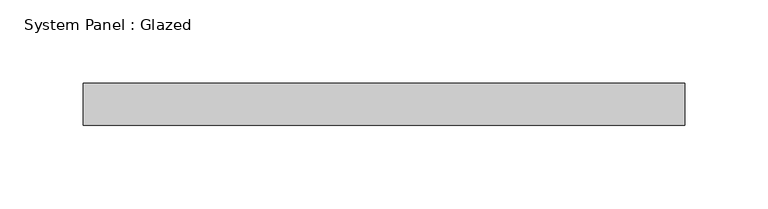
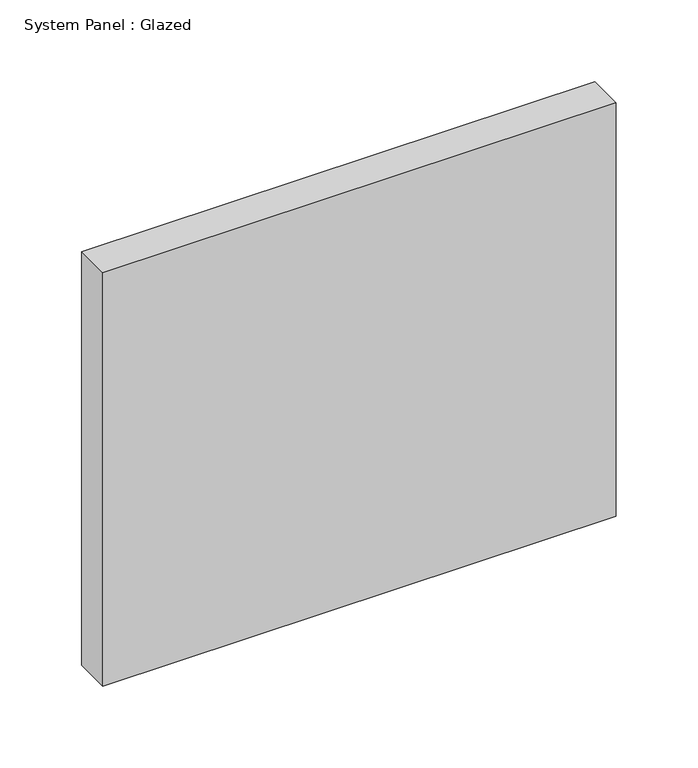
"""IFC4 building model written with IfcOpenShell, lengths in millimetres: plate geometry, System Panel : Glazed."""

from ifc_helpers import new_model, si_unit, origin, origin_with_axes, place, context, project, spatial, polyline, outline, extrude, source, transform, mapped, element, save


def system_panel_glazed_bcdea059(model_context):
    return source(origin(), model_context, "Body", "SweptSolid", [
        extrude(outline(polyline([(180.975, 19.05), (-180.975, 19.05), (-180.975, 44.45), (180.975, 44.45), (180.975, 19.05)])), origin_with_axes(), (0.0, 0.0, 1.0), 308.0546147),
    ])


if __name__ == "__main__":
    model = new_model("IFC4")
    model_context = context("Model", 3, world=origin())
    ifc_project = project(units=[si_unit("LENGTHUNIT", "METRE", prefix="MILLI")], contexts=[model_context])
    site = spatial("IfcSite", under=ifc_project)
    building = spatial("IfcBuilding", under=site)
    placement = place(None, origin())
    system_panel_glazed_shape = system_panel_glazed_bcdea059(model_context)
    element("IfcPlate", 1, ObjectType="System Panel : Glazed", at=placement, inside=building, context=model_context, shape_type="MappedRepresentation", body=[
        mapped(system_panel_glazed_shape, transform((0.0, 0.0, 0.0), x_axis=(1.0, 0.0, 0.0), y_axis=(0.0, 1.0, 0.0), z_axis=(0.0, 0.0, 1.0))),
    ])
    save(model, "model.ifc")

# Revit data of these elements
# Type "System Panel : Glazed"
#   Construction Type Id = "GSP4R"
#   Analytic Construction = "1/8 in Pilkington single glazing"
#   Visual Light Transmittance = 0.9
#   Solar Heat Gain Coefficient = 0.86
#   Heat Transfer Coefficient (U) = 1.18115 BTU/(h·ft²·°F)
#   Define Thermal Properties by = 1
# Element 1 (IfcPlate, "System Panel : Glazed")
#   Materials on its faces: "Glass"
# Materials
#   "Glass": class "Glass", colour RGB 0 128 192, transparency 0.75, Description = "Soda Lime Glass", Cost = 0
